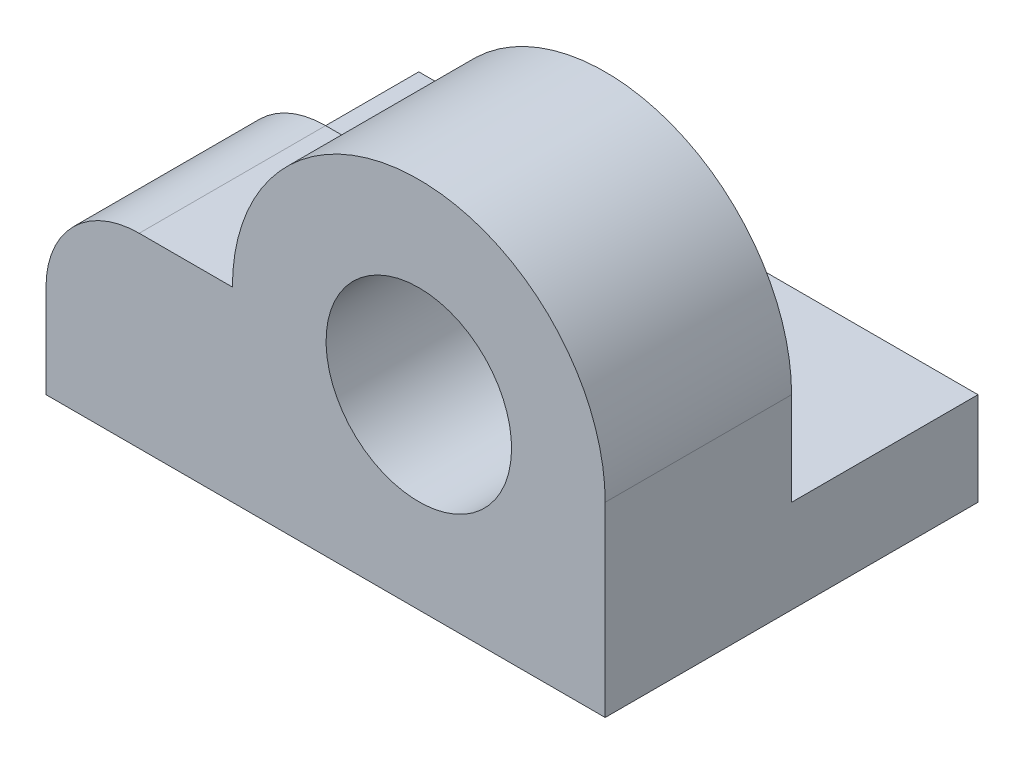
ISO-10303-21;
HEADER;
FILE_DESCRIPTION(('STEP AP214'),'2;1');
FILE_NAME('part.step','',(''),(''),'','','');
FILE_SCHEMA(('AUTOMOTIVE_DESIGN { 1 0 10303 214 1 1 1 1 }'));
ENDSEC;
DATA;
#1=APPLICATION_CONTEXT('core data for automotive mechanical design processes');
#2=APPLICATION_PROTOCOL_DEFINITION('international standard','automotive_design',2000,#1);
#3=PRODUCT_CONTEXT('',#1,'mechanical');
#4=PRODUCT('Part','Part','',(#3));
#5=PRODUCT_RELATED_PRODUCT_CATEGORY('part','',(#4));
#6=PRODUCT_DEFINITION_FORMATION('','',#4);
#7=PRODUCT_DEFINITION_CONTEXT('part definition',#1,'design');
#8=PRODUCT_DEFINITION('design','',#6,#7);
#9=PRODUCT_DEFINITION_SHAPE('','',#8);
#10=(LENGTH_UNIT() NAMED_UNIT(*) SI_UNIT(.MILLI.,.METRE.));
#11=(NAMED_UNIT(*) PLANE_ANGLE_UNIT() SI_UNIT($,.RADIAN.));
#12=(NAMED_UNIT(*) SI_UNIT($,.STERADIAN.) SOLID_ANGLE_UNIT());
#13=UNCERTAINTY_MEASURE_WITH_UNIT(LENGTH_MEASURE(1.E-05),#10,'distance_accuracy_value','');
#14=(GEOMETRIC_REPRESENTATION_CONTEXT(3) GLOBAL_UNCERTAINTY_ASSIGNED_CONTEXT((#13)) GLOBAL_UNIT_ASSIGNED_CONTEXT((#10,
#11,#12)) REPRESENTATION_CONTEXT('',''));
#15=CARTESIAN_POINT('',(0.,0.,0.));
#16=DIRECTION('',(0.,0.,1.));
#17=DIRECTION('',(1.,0.,0.));
#18=AXIS2_PLACEMENT_3D('',#15,#16,#17);
#19=CARTESIAN_POINT('',(30.,40.,0.));
#20=DIRECTION('',(0.,0.,-1.));
#21=DIRECTION('',(0.,1.,0.));
#22=AXIS2_PLACEMENT_3D('',#19,#20,#21);
#23=PLANE('',#22);
#24=CARTESIAN_POINT('',(10.,20.,0.));
#25=DIRECTION('',(0.,0.,-1.));
#26=DIRECTION('',(0.,1.,0.));
#27=AXIS2_PLACEMENT_3D('',#24,#25,#26);
#28=CIRCLE('',#27,9.95);
#29=CARTESIAN_POINT('',(10.,29.95,0.));
#30=VERTEX_POINT('',#29);
#31=EDGE_CURVE('E200',#30,#30,#28,.T.);
#32=ORIENTED_EDGE('',*,*,#31,.T.);
#33=EDGE_LOOP('',(#32));
#34=FACE_BOUND('',#33,.T.);
#35=CARTESIAN_POINT('',(-20.,9.99999999999997,0.));
#36=DIRECTION('',(0.,0.,-1.));
#37=DIRECTION('',(0.,1.,0.));
#38=AXIS2_PLACEMENT_3D('',#35,#36,#37);
#39=CIRCLE('',#38,10.);
#40=CARTESIAN_POINT('',(-30.,9.99999999999998,0.));
#41=VERTEX_POINT('',#40);
#42=CARTESIAN_POINT('',(-20.,20.,0.));
#43=VERTEX_POINT('',#42);
#44=EDGE_CURVE('E203',#41,#43,#39,.T.);
#45=ORIENTED_EDGE('',*,*,#44,.F.);
#46=DIRECTION('',(0.,-1.,0.));
#47=VECTOR('',#46,1.);
#48=CARTESIAN_POINT('',(-30.,40.,0.));
#49=LINE('',#48,#47);
#50=CARTESIAN_POINT('',(-30.,0.,0.));
#51=VERTEX_POINT('',#50);
#52=EDGE_CURVE('E151',#41,#51,#49,.T.);
#53=ORIENTED_EDGE('',*,*,#52,.T.);
#54=DIRECTION('',(-1.,0.,0.));
#55=VECTOR('',#54,1.);
#56=CARTESIAN_POINT('',(30.,0.,0.));
#57=LINE('',#56,#55);
#58=CARTESIAN_POINT('',(30.,0.,0.));
#59=VERTEX_POINT('',#58);
#60=EDGE_CURVE('E169',#59,#51,#57,.T.);
#61=ORIENTED_EDGE('',*,*,#60,.F.);
#62=DIRECTION('',(0.,-1.,0.));
#63=VECTOR('',#62,1.);
#64=CARTESIAN_POINT('',(30.,40.,0.));
#65=LINE('',#64,#63);
#66=CARTESIAN_POINT('',(30.,20.,0.));
#67=VERTEX_POINT('',#66);
#68=EDGE_CURVE('E112',#67,#59,#65,.T.);
#69=ORIENTED_EDGE('',*,*,#68,.F.);
#70=CARTESIAN_POINT('',(10.,20.,0.));
#71=DIRECTION('',(0.,0.,-1.));
#72=DIRECTION('',(0.,1.,0.));
#73=AXIS2_PLACEMENT_3D('',#70,#71,#72);
#74=CIRCLE('',#73,20.);
#75=CARTESIAN_POINT('',(-10.,20.,0.));
#76=VERTEX_POINT('',#75);
#77=EDGE_CURVE('E80',#76,#67,#74,.T.);
#78=ORIENTED_EDGE('',*,*,#77,.F.);
#79=DIRECTION('',(-1.,0.,0.));
#80=VECTOR('',#79,1.);
#81=CARTESIAN_POINT('',(30.,20.,0.));
#82=LINE('',#81,#80);
#83=EDGE_CURVE('E172',#76,#43,#82,.T.);
#84=ORIENTED_EDGE('',*,*,#83,.T.);
#85=EDGE_LOOP('',(#45,#53,#61,#69,#78,#84));
#86=FACE_BOUND('',#85,.T.);
#87=ADVANCED_FACE('F62',(#34,#86),#23,.F.);
#88=CARTESIAN_POINT('',(30.,9.99999999999999,-20.));
#89=DIRECTION('',(0.,0.,1.));
#90=DIRECTION('',(0.,-1.,0.));
#91=AXIS2_PLACEMENT_3D('',#88,#89,#90);
#92=PLANE('',#91);
#93=CARTESIAN_POINT('',(10.,20.,-20.));
#94=DIRECTION('',(0.,0.,-1.));
#95=DIRECTION('',(0.,1.,0.));
#96=AXIS2_PLACEMENT_3D('',#93,#94,#95);
#97=CIRCLE('',#96,9.95);
#98=CARTESIAN_POINT('',(10.,29.95,-20.));
#99=VERTEX_POINT('',#98);
#100=EDGE_CURVE('E211',#99,#99,#97,.T.);
#101=ORIENTED_EDGE('',*,*,#100,.F.);
#102=EDGE_LOOP('',(#101));
#103=FACE_BOUND('',#102,.T.);
#104=CARTESIAN_POINT('',(-20.,9.99999999999999,-20.));
#105=DIRECTION('',(0.,0.,-1.));
#106=DIRECTION('',(0.,1.,0.));
#107=AXIS2_PLACEMENT_3D('',#104,#105,#106);
#108=CIRCLE('',#107,10.);
#109=CARTESIAN_POINT('',(-30.,9.99999999999999,-20.));
#110=VERTEX_POINT('',#109);
#111=CARTESIAN_POINT('',(-20.,20.,-20.));
#112=VERTEX_POINT('',#111);
#113=EDGE_CURVE('E132',#110,#112,#108,.T.);
#114=ORIENTED_EDGE('',*,*,#113,.T.);
#115=DIRECTION('',(-1.,0.,0.));
#116=VECTOR('',#115,1.);
#117=CARTESIAN_POINT('',(0.,20.,-20.));
#118=LINE('',#117,#116);
#119=CARTESIAN_POINT('',(-10.,20.,-20.));
#120=VERTEX_POINT('',#119);
#121=EDGE_CURVE('E142',#120,#112,#118,.T.);
#122=ORIENTED_EDGE('',*,*,#121,.F.);
#123=CARTESIAN_POINT('',(10.,20.,-20.));
#124=DIRECTION('',(0.,0.,-1.));
#125=DIRECTION('',(0.,1.,0.));
#126=AXIS2_PLACEMENT_3D('',#123,#124,#125);
#127=CIRCLE('',#126,20.);
#128=CARTESIAN_POINT('',(30.,20.,-20.));
#129=VERTEX_POINT('',#128);
#130=EDGE_CURVE('E171',#120,#129,#127,.T.);
#131=ORIENTED_EDGE('',*,*,#130,.T.);
#132=DIRECTION('',(0.,1.,0.));
#133=VECTOR('',#132,1.);
#134=CARTESIAN_POINT('',(30.,9.99999999999999,-20.));
#135=LINE('',#134,#133);
#136=CARTESIAN_POINT('',(30.,9.99999999999999,-20.));
#137=VERTEX_POINT('',#136);
#138=EDGE_CURVE('E159',#137,#129,#135,.T.);
#139=ORIENTED_EDGE('',*,*,#138,.F.);
#140=DIRECTION('',(-1.,0.,0.));
#141=VECTOR('',#140,1.);
#142=CARTESIAN_POINT('',(30.,9.99999999999999,-20.));
#143=LINE('',#142,#141);
#144=EDGE_CURVE('E152',#137,#110,#143,.T.);
#145=ORIENTED_EDGE('',*,*,#144,.T.);
#146=EDGE_LOOP('',(#114,#122,#131,#139,#145));
#147=FACE_BOUND('',#146,.T.);
#148=ADVANCED_FACE('F158',(#103,#147),#92,.F.);
#149=CARTESIAN_POINT('',(30.,0.,0.));
#150=DIRECTION('',(0.,1.,0.));
#151=DIRECTION('',(0.,0.,1.));
#152=AXIS2_PLACEMENT_3D('',#149,#150,#151);
#153=PLANE('',#152);
#154=DIRECTION('',(0.,0.,-1.));
#155=VECTOR('',#154,1.);
#156=CARTESIAN_POINT('',(-30.,0.,0.));
#157=LINE('',#156,#155);
#158=CARTESIAN_POINT('',(-30.,0.,-40.));
#159=VERTEX_POINT('',#158);
#160=EDGE_CURVE('E225',#51,#159,#157,.T.);
#161=ORIENTED_EDGE('',*,*,#160,.T.);
#162=DIRECTION('',(-1.,0.,0.));
#163=VECTOR('',#162,1.);
#164=CARTESIAN_POINT('',(30.,0.,-40.));
#165=LINE('',#164,#163);
#166=CARTESIAN_POINT('',(30.,0.,-40.));
#167=VERTEX_POINT('',#166);
#168=EDGE_CURVE('E165',#167,#159,#165,.T.);
#169=ORIENTED_EDGE('',*,*,#168,.F.);
#170=DIRECTION('',(0.,0.,-1.));
#171=VECTOR('',#170,1.);
#172=CARTESIAN_POINT('',(30.,0.,0.));
#173=LINE('',#172,#171);
#174=EDGE_CURVE('E216',#59,#167,#173,.T.);
#175=ORIENTED_EDGE('',*,*,#174,.F.);
#176=ORIENTED_EDGE('',*,*,#60,.T.);
#177=EDGE_LOOP('',(#161,#169,#175,#176));
#178=FACE_BOUND('',#177,.T.);
#179=ADVANCED_FACE('F192',(#178),#153,.F.);
#180=CARTESIAN_POINT('',(30.,0.,-40.));
#181=DIRECTION('',(0.,0.,1.));
#182=DIRECTION('',(0.,-1.,0.));
#183=AXIS2_PLACEMENT_3D('',#180,#181,#182);
#184=PLANE('',#183);
#185=DIRECTION('',(0.,1.,0.));
#186=VECTOR('',#185,1.);
#187=CARTESIAN_POINT('',(-30.,0.,-40.));
#188=LINE('',#187,#186);
#189=CARTESIAN_POINT('',(-30.,10.,-40.));
#190=VERTEX_POINT('',#189);
#191=EDGE_CURVE('E104',#159,#190,#188,.T.);
#192=ORIENTED_EDGE('',*,*,#191,.T.);
#193=DIRECTION('',(-1.,0.,0.));
#194=VECTOR('',#193,1.);
#195=CARTESIAN_POINT('',(30.,10.,-40.));
#196=LINE('',#195,#194);
#197=CARTESIAN_POINT('',(30.,10.,-40.));
#198=VERTEX_POINT('',#197);
#199=EDGE_CURVE('E156',#198,#190,#196,.T.);
#200=ORIENTED_EDGE('',*,*,#199,.F.);
#201=DIRECTION('',(0.,1.,0.));
#202=VECTOR('',#201,1.);
#203=CARTESIAN_POINT('',(30.,0.,-40.));
#204=LINE('',#203,#202);
#205=EDGE_CURVE('E217',#167,#198,#204,.T.);
#206=ORIENTED_EDGE('',*,*,#205,.F.);
#207=ORIENTED_EDGE('',*,*,#168,.T.);
#208=EDGE_LOOP('',(#192,#200,#206,#207));
#209=FACE_BOUND('',#208,.T.);
#210=ADVANCED_FACE('F184',(#209),#184,.F.);
#211=CARTESIAN_POINT('',(30.,10.,-40.));
#212=DIRECTION('',(0.,-1.,0.));
#213=DIRECTION('',(0.,0.,-1.));
#214=AXIS2_PLACEMENT_3D('',#211,#212,#213);
#215=PLANE('',#214);
#216=DIRECTION('',(0.,0.,1.));
#217=VECTOR('',#216,1.);
#218=CARTESIAN_POINT('',(-30.,10.,-40.));
#219=LINE('',#218,#217);
#220=EDGE_CURVE('E149',#190,#110,#219,.T.);
#221=ORIENTED_EDGE('',*,*,#220,.T.);
#222=ORIENTED_EDGE('',*,*,#144,.F.);
#223=DIRECTION('',(0.,0.,1.));
#224=VECTOR('',#223,1.);
#225=CARTESIAN_POINT('',(30.,10.,-40.));
#226=LINE('',#225,#224);
#227=EDGE_CURVE('E88',#198,#137,#226,.T.);
#228=ORIENTED_EDGE('',*,*,#227,.F.);
#229=ORIENTED_EDGE('',*,*,#199,.T.);
#230=EDGE_LOOP('',(#221,#222,#228,#229));
#231=FACE_BOUND('',#230,.T.);
#232=ADVANCED_FACE('F153',(#231),#215,.F.);
#233=CARTESIAN_POINT('',(30.,0.,0.));
#234=DIRECTION('',(1.,0.,0.));
#235=DIRECTION('',(0.,0.,-1.));
#236=AXIS2_PLACEMENT_3D('',#233,#234,#235);
#237=PLANE('',#236);
#238=DIRECTION('',(0.,0.,-1.));
#239=VECTOR('',#238,1.);
#240=CARTESIAN_POINT('',(30.,20.,40.));
#241=LINE('',#240,#239);
#242=EDGE_CURVE('E66',#67,#129,#241,.T.);
#243=ORIENTED_EDGE('',*,*,#242,.F.);
#244=ORIENTED_EDGE('',*,*,#68,.T.);
#245=ORIENTED_EDGE('',*,*,#174,.T.);
#246=ORIENTED_EDGE('',*,*,#205,.T.);
#247=ORIENTED_EDGE('',*,*,#227,.T.);
#248=ORIENTED_EDGE('',*,*,#138,.T.);
#249=EDGE_LOOP('',(#243,#244,#245,#246,#247,#248));
#250=FACE_BOUND('',#249,.T.);
#251=ADVANCED_FACE('F174',(#250),#237,.T.);
#252=CARTESIAN_POINT('',(-30.,0.,0.));
#253=DIRECTION('',(1.,0.,0.));
#254=DIRECTION('',(0.,0.,-1.));
#255=AXIS2_PLACEMENT_3D('',#252,#253,#254);
#256=PLANE('',#255);
#257=ORIENTED_EDGE('',*,*,#52,.F.);
#258=DIRECTION('',(0.,0.,-1.));
#259=VECTOR('',#258,1.);
#260=CARTESIAN_POINT('',(-30.,9.99999999999995,40.));
#261=LINE('',#260,#259);
#262=EDGE_CURVE('E12',#41,#110,#261,.T.);
#263=ORIENTED_EDGE('',*,*,#262,.T.);
#264=ORIENTED_EDGE('',*,*,#220,.F.);
#265=ORIENTED_EDGE('',*,*,#191,.F.);
#266=ORIENTED_EDGE('',*,*,#160,.F.);
#267=EDGE_LOOP('',(#257,#263,#264,#265,#266));
#268=FACE_BOUND('',#267,.T.);
#269=ADVANCED_FACE('F146',(#268),#256,.F.);
#270=CARTESIAN_POINT('',(10.,20.,40.));
#271=DIRECTION('',(0.,0.,-1.));
#272=DIRECTION('',(0.,1.,0.));
#273=AXIS2_PLACEMENT_3D('',#270,#271,#272);
#274=CYLINDRICAL_SURFACE('',#273,9.95);
#275=ORIENTED_EDGE('',*,*,#100,.T.);
#276=EDGE_LOOP('',(#275));
#277=FACE_BOUND('',#276,.T.);
#278=ORIENTED_EDGE('',*,*,#31,.F.);
#279=EDGE_LOOP('',(#278));
#280=FACE_BOUND('',#279,.T.);
#281=ADVANCED_FACE('F185',(#277,#280),#274,.F.);
#282=CARTESIAN_POINT('',(10.,20.,40.));
#283=DIRECTION('',(0.,0.,-1.));
#284=DIRECTION('',(0.,1.,0.));
#285=AXIS2_PLACEMENT_3D('',#282,#283,#284);
#286=CYLINDRICAL_SURFACE('',#285,20.);
#287=ORIENTED_EDGE('',*,*,#77,.T.);
#288=ORIENTED_EDGE('',*,*,#242,.T.);
#289=ORIENTED_EDGE('',*,*,#130,.F.);
#290=DIRECTION('',(0.,0.,-1.));
#291=VECTOR('',#290,1.);
#292=CARTESIAN_POINT('',(-10.,20.,40.));
#293=LINE('',#292,#291);
#294=EDGE_CURVE('E206',#76,#120,#293,.T.);
#295=ORIENTED_EDGE('',*,*,#294,.F.);
#296=EDGE_LOOP('',(#287,#288,#289,#295));
#297=FACE_BOUND('',#296,.T.);
#298=ADVANCED_FACE('F168',(#297),#286,.T.);
#299=CARTESIAN_POINT('',(0.,20.,40.));
#300=DIRECTION('',(0.,-1.,0.));
#301=DIRECTION('',(0.,0.,-1.));
#302=AXIS2_PLACEMENT_3D('',#299,#300,#301);
#303=PLANE('',#302);
#304=ORIENTED_EDGE('',*,*,#294,.T.);
#305=ORIENTED_EDGE('',*,*,#121,.T.);
#306=DIRECTION('',(0.,0.,-1.));
#307=VECTOR('',#306,1.);
#308=CARTESIAN_POINT('',(-20.,20.,40.));
#309=LINE('',#308,#307);
#310=EDGE_CURVE('E139',#43,#112,#309,.T.);
#311=ORIENTED_EDGE('',*,*,#310,.F.);
#312=ORIENTED_EDGE('',*,*,#83,.F.);
#313=EDGE_LOOP('',(#304,#305,#311,#312));
#314=FACE_BOUND('',#313,.T.);
#315=ADVANCED_FACE('F230',(#314),#303,.F.);
#316=CARTESIAN_POINT('',(-20.,9.99999999999995,40.));
#317=DIRECTION('',(0.,0.,-1.));
#318=DIRECTION('',(0.,1.,0.));
#319=AXIS2_PLACEMENT_3D('',#316,#317,#318);
#320=CYLINDRICAL_SURFACE('',#319,10.);
#321=ORIENTED_EDGE('',*,*,#44,.T.);
#322=ORIENTED_EDGE('',*,*,#310,.T.);
#323=ORIENTED_EDGE('',*,*,#113,.F.);
#324=ORIENTED_EDGE('',*,*,#262,.F.);
#325=EDGE_LOOP('',(#321,#322,#323,#324));
#326=FACE_BOUND('',#325,.T.);
#327=ADVANCED_FACE('F133',(#326),#320,.T.);
#328=CLOSED_SHELL('',(#87,#148,#179,#210,#232,#251,#269,#281,#298,#315,#327));
#329=MANIFOLD_SOLID_BREP('B2',#328);
#330=ADVANCED_BREP_SHAPE_REPRESENTATION('',(#18,#329),#14);
#331=SHAPE_DEFINITION_REPRESENTATION(#9,#330);
ENDSEC;
END-ISO-10303-21;
